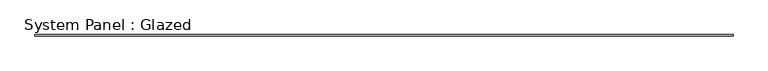
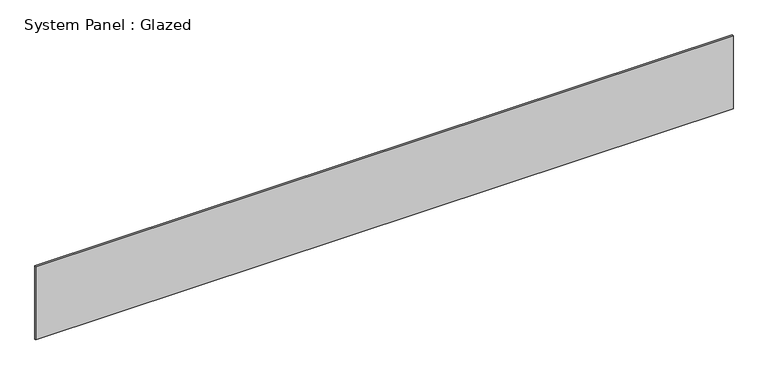
"""IFC4 building model written with IfcOpenShell, lengths in millimetres: plate geometry, System Panel : Glazed."""

from ifc_helpers import new_model, si_unit, origin, origin_with_axes, place, context, project, spatial, polyline, outline, extrude, source, transform, mapped, element, save


def system_panel_glazed_9c6e7784(model_context):
    return source(origin(), model_context, "Body", "SweptSolid", [
        extrude(outline(polyline([(6857.135375, 19.05), (-6857.135375, 19.05), (-6857.135375, 44.45), (6857.135375, 44.45), (6857.135375, 19.05)])), origin_with_axes(), (0.0, 0.0, 1.0), 1524.0),
    ])


if __name__ == "__main__":
    model = new_model("IFC4")
    model_context = context("Model", 3, world=origin())
    ifc_project = project(units=[si_unit("LENGTHUNIT", "METRE", prefix="MILLI")], contexts=[model_context])
    site = spatial("IfcSite", under=ifc_project)
    building = spatial("IfcBuilding", under=site)
    placement = place(None, origin())
    system_panel_glazed_shape = system_panel_glazed_9c6e7784(model_context)
    element("IfcPlate", 1, ObjectType="System Panel : Glazed", at=placement, inside=building, context=model_context, shape_type="MappedRepresentation", body=[
        mapped(system_panel_glazed_shape, transform((0.0, 0.0, 0.0), x_axis=(1.0, 0.0, 0.0), y_axis=(0.0, 1.0, 0.0), z_axis=(0.0, 0.0, 1.0))),
    ])
    save(model, "model.ifc")

# Revit data of these elements
# Type "System Panel : Glazed"
#   Construction Type Id = "GSP4R"
#   Analytic Construction = "1/8 in Pilkington single glazing"
#   Visual Light Transmittance = 0.9
#   Solar Heat Gain Coefficient = 0.86
#   Heat Transfer Coefficient (U) = 1.18115 BTU/(h·ft²·°F)
# Element 1 (IfcPlate, "System Panel : Glazed")
#   Materials on its faces: "Glass"
# Materials
#   "Glass": class "Glass", colour RGB 0 128 192, transparency 0.75, Description = "Soda Lime Glass", Cost = 0
